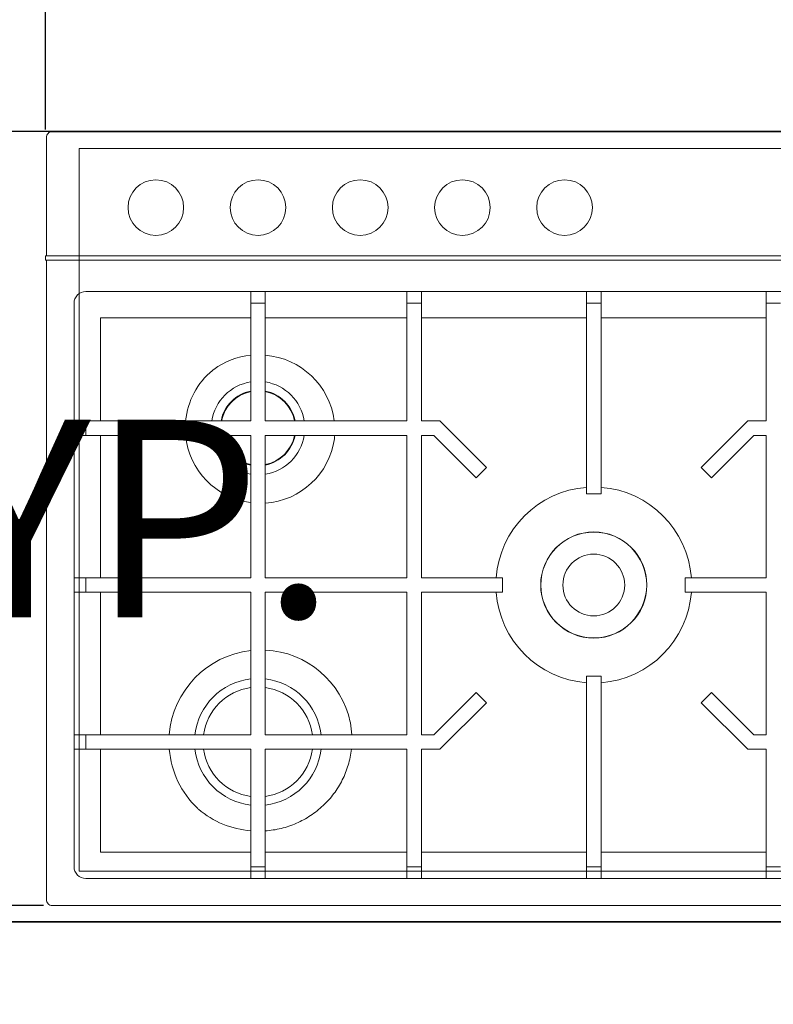
# Model space of a CAD drawing. Units: inches. Extents: x -1198 to -69, y -512 to 437.
# Tile 7 of 50: x -979 to -956, y 159 to 189. Entities that reach past the tile are written whole.
import ezdxf

# ---------------------------------------------------------------- set-up
doc = ezdxf.new("R2010")
doc.units = ezdxf.units.IN
doc.header["$MEASUREMENT"] = 0
for name, color, linetype, lineweight in [('0_Pen_No__7', 7, 'Continuous', 18), ('A-ANNO-DIMS', 2, 'Continuous', 18), ('A-EQPM', 60, 'Continuous', 18), ('A-FLOR-CASE', 7, 'Continuous', 25), ('A-WALL', 7, 'Continuous', 35)]:
    doc.layers.add(name, color=color, linetype=linetype, lineweight=lineweight)
doc.styles.get("Standard").update_dxf_attribs({"font": 'arial.ttf'})
doc.dimstyles.get("Standard").update_dxf_attribs({"dimtxt": 6, "dimasz": 6, "dimexe": 0.18, "dimexo": 0.0625, "dimgap": 0.09, "dimtad": 0, "dimtih": 1, "dimtoh": 1, "dimdec": 0, "dimzin": 0, "dimdsep": 46, "dimlunit": 4, "dimtxsty": 'Standard', "dimblk": 'OBLIQUE', "dimcen": 0.09, "dimadec": 0, "dimazin": 0, "dimtfac": 1, "dimtdec": 0, "dimtofl": 0, "dimtmove": 0, "dimatfit": 3, "dimfxl": 1, "dimtolj": 1, "dimtzin": 0, "dimarcsym": 0})

# ---------------------------------------------------------------- blocks, each defined once
blk = doc.blocks.new('new block')
at = {"layer": '0_Pen_No__7'}
for p, q in [((-80.82, 567.06), (-69.55, 567.06)), ((68.97, 567.06), (57.71, 567.06)), ((207.5, 567.06), (196.24, 567.06)), ((328.01, 567.06), (316.75, 567.06)), ((-69.55, 555.8), (57.71, 555.8)), ((196.24, 555.8), (68.97, 555.8)), ((316.75, 555.8), (207.5, 555.8)), ((444.01, 555.8), (328.01, 555.8)), ((444.01, 476.4), (444.01, 555.8)), ((455.27, 465.14), (455.27, 476.4)), ((444.01, 355.33), (444.01, 465.14)), ((455.27, 344.07), (455.27, 355.33)), ((444.01, 344.07), (444.01, 234.26)), ((455.27, 234.26), (455.27, 223)), ((-69.55, 143.6), (57.71, 143.6)), ((196.24, 143.6), (68.97, 143.6)), ((316.75, 143.6), (207.5, 143.6)), ((-80.82, 132.33), (-69.55, 132.33)), ((57.71, 132.33), (68.97, 132.33)), ((207.5, 132.33), (196.24, 132.33)), ((328.01, 132.33), (316.75, 132.33)), ((-359, 99.11), (485.68, 99.11)), ((485.68, 95.73), (-359, 95.73))]:
    blk.add_line(p, q, dxfattribs=at)
for points in [[(-354.49, 596.91), (481.18, 596.91, -0.414214), (485.68, 592.4), (485.68, 99.11), (486.24, 99.11), (486.24, 95.73), (485.68, 95.73), (485.68, 4.5, -0.414214), (481.18, 0), (-354.49, 0, -0.414214), (-359, 4.5), (-359, 95.73), (-359.56, 95.73), (-359.56, 99.11), (-359, 99.11), (-359, 592.4, -0.414214)], [(464.28, 132.33), (464.28, 567.06, 0.414214), (455.27, 576.07), (-328.59, 576.07, 0.414214), (-337.6, 567.06), (-337.6, 132.33, 0.414214), (-328.59, 123.32), (455.27, 123.32, 0.414214)]]:
    blk.add_lwpolyline(points, format="xyb", close=True, dxfattribs=at)
for points in [[(-333.7, 12.95), (460.3, 12.95), (460.3, 570.44), (-333.7, 570.44)], [(207.5, 465.14), (207.5, 355.33), (316.75, 355.33), (316.75, 465.14)], [(316.75, 234.26), (207.5, 234.26), (207.5, 344.07), (316.75, 344.07)]]:
    blk.add_lwpolyline(points, close=True, dxfattribs=at)
for points in [[(-69.55, 576.07), (-69.55, 476.4), (-55.4, 476.4), (-19.45, 440.45), (-27.41, 432.48), (-60.06, 465.14), (-69.55, 465.14), (-69.55, 355.33), (-7.05, 355.33), (-7.05, 344.07), (-69.55, 344.07), (-69.55, 234.26), (-60.06, 234.26), (-27.41, 266.91), (-19.45, 258.94), (-55.4, 223), (-69.55, 223), (-69.55, 123.32)], [(57.71, 576.07), (57.71, 420.09), (68.97, 420.09), (68.97, 576.07)], [(196.24, 123.32), (196.24, 223), (182.08, 223), (146.13, 258.94), (154.09, 266.91), (186.75, 234.26), (196.24, 234.26), (196.24, 344.07), (133.73, 344.07), (133.73, 355.33), (196.24, 355.33), (196.24, 465.14), (186.75, 465.14), (154.09, 432.48), (146.13, 440.45), (182.08, 476.4), (196.24, 476.4), (196.24, 576.07)], [(207.5, 576.07), (207.5, 476.4), (316.75, 476.4), (316.75, 576.07)], [(328.01, 576.07), (328.01, 476.4), (464.28, 476.4)], [(316.75, 539.36), (315.2, 539.23), (313.66, 539.07), (312.12, 538.88), (310.58, 538.65), (309.05, 538.4), (307.53, 538.1), (306.01, 537.78), (304.5, 537.42), (303, 537.04), (301.5, 536.62), (300.02, 536.16), (298.55, 535.68), (297.08, 535.17), (295.63, 534.62), (294.19, 534.05), (292.76, 533.44), (291.35, 532.8), (289.95, 532.14), (288.56, 531.44), (287.19, 530.71), (285.84, 529.96), (284.5, 529.18), (283.18, 528.36), (281.87, 527.52), (280.59, 526.66), (279.32, 525.76), (278.07, 524.84), (276.85, 523.89), (275.64, 522.92), (274.45, 521.92), (273.29, 520.89), (272.15, 519.84), (271.03, 518.76), (269.94, 517.67), (268.87, 516.54), (267.82, 515.4), (266.8, 514.23), (265.8, 513.04), (264.83, 511.83), (263.89, 510.6), (262.98, 509.35), (262.09, 508.08), (261.23, 506.78), (260.4, 505.47), (259.6, 504.15), (258.82, 502.8), (258.08, 501.44), (257.37, 500.06), (256.69, 498.67), (256.03, 497.26), (255.41, 495.84), (254.83, 494.41), (254.27, 492.96), (253.75, 491.5), (253.25, 490.03), (252.8, 488.55), (252.37, 487.05), (251.98, 485.55), (251.62, 484.04), (251.29, 482.53), (251, 481), (250.75, 479.47), (250.53, 477.94), (250.34, 476.4)], [(464.28, 465.14), (328.01, 465.14), (328.01, 355.33), (464.28, 355.33)], [(464.28, 234.26), (328.01, 234.26), (328.01, 344.07), (464.28, 344.07)], [(68.97, 123.32), (68.97, 279.31), (57.71, 279.31), (57.71, 123.32)], [(207.5, 123.32), (207.5, 223), (316.75, 223), (316.75, 123.32)], [(328.01, 123.32), (328.01, 223), (464.28, 223)], [(444.01, 223), (444.01, 143.6), (328.01, 143.6)]]:
    blk.add_lwpolyline(points, dxfattribs=at)
for centre, radius in [((63.34, 349.7), 40.95), ((63.34, 349.7), 40.83), ((63.34, 349.7), 23.84), ((85.87, 58.56), 21.45), ((164.7, 58.56), 21.45), ((243.54, 58.56), 21.45), ((322.38, 58.56), 21.45), ((401.21, 58.56), 21.45)]:
    blk.add_circle(centre, radius, dxfattribs=at)
for centre, radius, start, end in [((322.14, 468.12), 71.42, 49.7275, 85.28931), ((322.38, 470.77), 48.99, 96.60065, 173.39935), ((322.38, 470.77), 48.99, 6.60065, 83.39935), ((355.62, 507.66), 19.61, 46.47207, 49.65802), ((320.47, 470.71), 70.6, 4.62083, 46.44687), ((322.38, 470.77), 42.35, 97.64264, 172.3569), ((322.38, 470.77), 42.35, 7.6431, 82.35736), ((319.41, 468.81), 69.49, 183.03105, 190.60746), ((322.38, 470.77), 48.99, 186.60065, 263.39935), ((322.38, 470.77), 42.35, 187.6431, 262.35736), ((320.15, 470.72), 70.94, 276.3643, 355.48211), ((322.38, 470.77), 48.99, 276.60065, 353.39935), ((322.38, 470.77), 42.35, 277.64264, 352.3569), ((269.57, 459.48), 18.78, 190.60771, 191.88529), ((319.99, 470.1), 70.32, 191.89609, 267.35247), ((63.34, 349.7), 75.53, 94.27701, 175.72431), ((63.34, 349.7), 75.53, 4.27569, 85.72299), ((63.34, 349.7), 75.53, 184.27569, 265.72299), ((63.34, 349.7), 75.53, 274.27701, 355.72431), ((320.48, 229.1), 57.52, 93.72225, 172.22668), ((320.57, 228.68), 57.95, 5.52347, 82.62478), ((322.38, 228.63), 36.04, 98.99031, 171.00966), ((322.38, 228.63), 36.04, 8.99034, 81.00969), ((322.38, 228.63), 29.08, 101.17283, 168.8339), ((322.38, 228.63), 28.72, 101.31905, 168.69126), ((322.38, 228.63), 29.08, 11.1661, 78.82717), ((322.38, 228.63), 28.72, 11.30874, 78.68095), ((320.24, 230.21), 57.15, 173.81232, 175.93921), ((281.76, 234.38), 18.44, 172.21689, 173.81535), ((321.61, 230.78), 58.58, 187.63711, 265.23442), ((322.38, 228.63), 36.04, 188.99034, 261.00969), ((322.38, 228.63), 29.08, 191.1661, 258.82717), ((322.38, 228.63), 28.72, 191.30874, 258.68095), ((322.38, 228.63), 36.04, 278.99031, 351.00966), ((322.38, 228.63), 29.08, 281.17283, 348.8339), ((322.38, 228.63), 28.72, 281.31905, 348.69126), ((320.83, 228.69), 57.68, 309.3686, 354.33417), ((322.04, 230.74), 58.56, 275.84718, 306.13795), ((345.26, 198.93), 19.18, 306.17281, 309.34365)]:
    blk.add_arc(centre, radius, start, end, dxfattribs=at)
blk = doc.blocks.new('COUNTER-L')
at = {"ltscale": 10}
blk.add_line((49.349, 24), (0, 24), dxfattribs=at)
blk = doc.blocks.new('_Oblique')
at = {"color": 0, "linetype": 'ByBlock', "lineweight": -2}
blk.add_line((-0.5, -0.5), (0.5, 0.5), dxfattribs=at)
blk = doc.blocks.new('*D50')
at = {"layer": 'A-ANNO-DIMS', "color": 0, "lineweight": -2, "ltscale": 10, "transparency": 16777216}
for p, q in [((-978.462, 190.223), (-984.462, 190.223)), ((-978.462, 185.29), (-978.462, 190.403)), ((-945.163, 190.223), (-978.462, 190.223)), ((-945.163, 185.29), (-945.163, 190.403))]:
    blk.add_line(p, q, dxfattribs=at)
at = {"layer": 'DEFPOINTS', "color": 0, "ltscale": 10, "transparency": 16777216}
for p in [(-978.462, 190.223), (-978.462, 185.228), (-945.163, 185.228)]:
    blk.add_point(p, dxfattribs=at)
at = {"layer": 'A-ANNO-DIMS', "color": 0, "lineweight": -2, "ltscale": 10, "transparency": 16777216, "xscale": 6, "yscale": 6, "zscale": 6, "rotation": 180}
blk.add_blockref('_Oblique', (-978.462, 190.223), dxfattribs=at)
at = {"layer": 'A-ANNO-DIMS', "color": 0, "lineweight": -2, "ltscale": 10, "transparency": 16777216, "xscale": 6, "yscale": 6, "zscale": 6}
blk.add_blockref('_Oblique', (-945.163, 190.223), dxfattribs=at)
at = {"layer": 'A-ANNO-DIMS', "color": 0, "ltscale": 10, "transparency": 16777216, "insert": (-1009.24, 190.223), "char_height": 6, "attachment_point": 5}
blk.add_mtext('\\A1;HOB 33 TYP.', dxfattribs=at)
blk = doc.blocks.new('*D51')
at = {"layer": 'A-ANNO-DIMS', "color": 0, "lineweight": -2, "ltscale": 10, "transparency": 16777216}
for p, q in [((-978.525, 185.228), (-983.637, 185.228)), ((-983.457, 185.228), (-983.457, 176.582)), ((-983.457, 161.727), (-983.457, 170.373)), ((-978.525, 161.727), (-983.637, 161.727))]:
    blk.add_line(p, q, dxfattribs=at)
at = {"layer": 'DEFPOINTS', "color": 0, "ltscale": 10, "transparency": 16777216}
for p in [(-978.462, 185.228), (-983.457, 161.727), (-978.462, 161.727)]:
    blk.add_point(p, dxfattribs=at)
at = {"layer": 'A-ANNO-DIMS', "color": 0, "lineweight": -2, "ltscale": 10, "transparency": 16777216, "xscale": 6, "yscale": 6, "zscale": 6}
for p, rotation in [((-983.457, 185.228), 90), ((-983.457, 161.727), 270)]:
    blk.add_blockref('_Oblique', p, dxfattribs=dict(at, rotation=rotation))
at = {"layer": 'A-ANNO-DIMS', "color": 0, "ltscale": 10, "transparency": 16777216, "insert": (-983.457, 173.478), "char_height": 6, "attachment_point": 5}
blk.add_mtext('\\A1;24 TYP.', dxfattribs=at)

msp = doc.modelspace()

# ---------------------------------------------------------------- linework, layer by layer
at = {"layer": 'A-WALL', "ltscale": 10}
msp.add_line((-886.7509, 161.2277), (-1012.7509, 161.2277), dxfattribs=at)

# ---------------------------------------------------------------- block references
at = {"layer": 'A-EQPM', "xscale": 0.0393700787401575, "yscale": 0.0393700787401575, "zscale": 0.0393700787401575, "rotation": 180}
msp.add_blockref('new block', (-959.3186, 185.2277), dxfattribs=at)
at = {"layer": 'A-FLOR-CASE'}
msp.add_blockref('COUNTER-L', (-988.751, 161.228), dxfattribs=at)

# ---------------------------------------------------------------- dimensions: what is measured, and where the dimension line sits
at = {"layer": 'A-ANNO-DIMS', "ltscale": 10}
for base, p1, p2, angle, text, picture, middle in [((-978.4621, 190.2226), (-945.1627, 185.2277), (-978.4621, 185.2277), 180, 'HOB <> TYP.', '*D50', (-1009.2397, 190.2226)), ((-983.457, 161.7274), (-978.4621, 185.2277), (-978.4621, 161.7274), 270, '<> TYP.', '*D51', (-983.457, 173.4775))]:
    dim = msp.add_linear_dim(base=base, p1=p1, p2=p2, angle=angle, text=text, dimstyle='Standard', override={"dimdec": 0, "dimlfac": 1, "dimrnd": 0, "dimzin": 0, "dimdsep": 46, "dimlunit": 2}, dxfattribs=at)
    dim.commit()
    dim.dimension.update_dxf_attribs({"geometry": picture, "text_midpoint": middle})

doc.saveas('drawing.dxf')
